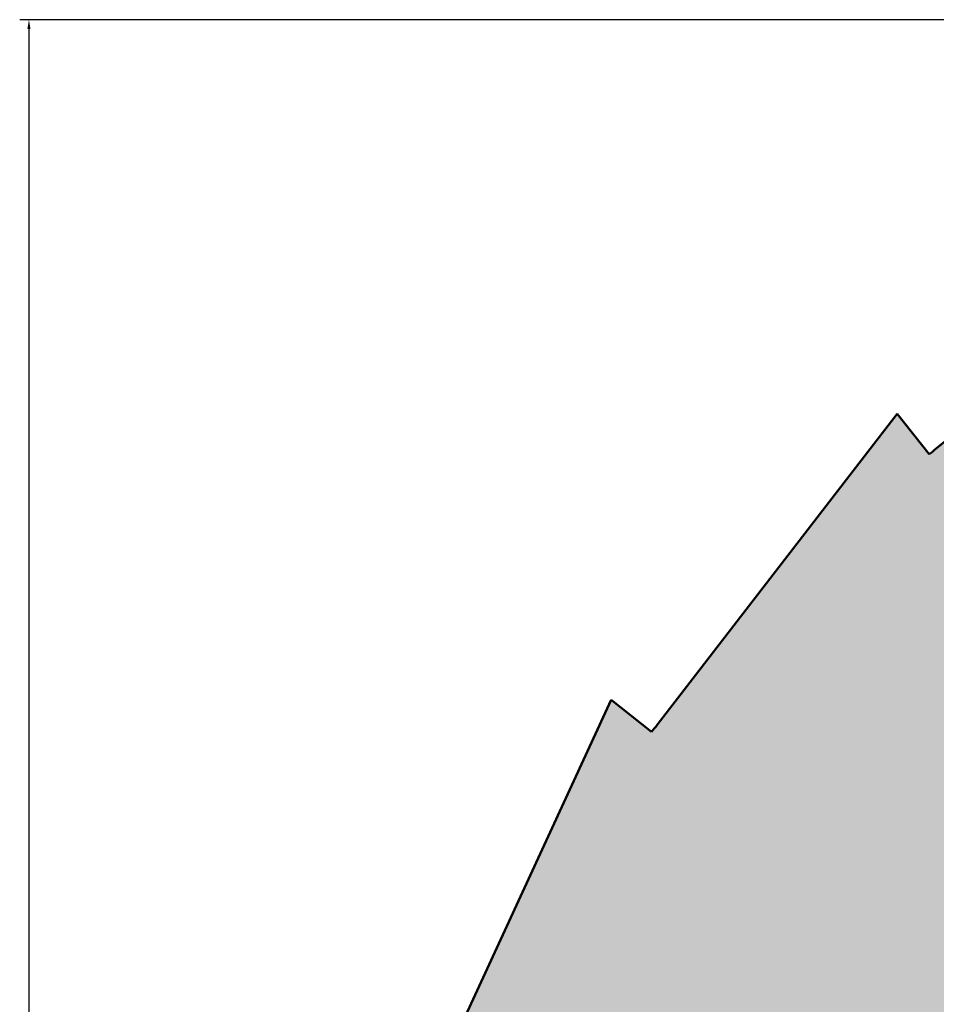
# Model space of a CAD drawing. Units: millimetres. Extents: x 2943.6 to 3032.7, y 1562 to 1639.7.
# Tile 4 of 9: x 2943.6 to 2961.4, y 1616.8 to 1635.8. Entities that reach past the tile are written whole.
import ezdxf

# ---------------------------------------------------------------- set-up
doc = ezdxf.new("R2010")
doc.units = ezdxf.units.MM
doc.layers.add('M-DIMS', color=2, linetype='Continuous', lineweight=18)
doc.layers.add('M-OUTL', color=7, linetype='Continuous', lineweight=50)
doc.layers.add('M-HATC', color=7, linetype='Continuous', lineweight=18, true_color=0xffffff)
doc.styles.get("Standard").update_dxf_attribs({"font": 'arial.ttf'})
doc.dimstyles.get("Standard").update_dxf_attribs({"dimtxt": 0.18, "dimasz": 0.18, "dimexe": 0.18, "dimexo": 0.0625, "dimgap": 0.09, "dimtad": 0, "dimtih": 1, "dimtoh": 1, "dimdec": 4, "dimzin": 0, "dimdsep": 46, "dimtxsty": 'Standard', "dimcen": 0.09, "dimadec": 0, "dimazin": 0, "dimtfac": 1, "dimtdec": 4, "dimtofl": 0, "dimtmove": 0, "dimatfit": 3, "dimfxl": 1, "dimtolj": 1, "dimtzin": 0, "dimarcsym": 0})

# ---------------------------------------------------------------- blocks, each defined once
blk = doc.blocks.new('*D4')
at = {"layer": 'Defpoints', "color": 0, "transparency": 16777216}
for p in [(2943.819, 1635.848), (2982.469, 1635.848), (2982.469, 1565.848)]:
    blk.add_point(p, dxfattribs=at)
at = {"layer": 'M-DIMS', "color": 0, "lineweight": -2, "transparency": 16777216}
for p, q in [((2982.407, 1635.848), (2943.639, 1635.848)), ((2943.819, 1635.668), (2943.819, 1601.03)), ((2943.819, 1566.028), (2943.819, 1600.666)), ((2982.407, 1565.848), (2943.639, 1565.848))]:
    blk.add_line(p, q, dxfattribs=at)
at = {"layer": 'M-DIMS', "color": 0, "transparency": 16777216}
for points in [[(2943.789, 1635.668), (2943.849, 1635.668), (2943.819, 1635.848)], [(2943.789, 1566.028), (2943.849, 1566.028), (2943.819, 1565.848)]]:
    blk.add_solid(points, dxfattribs=at)
at = {"layer": 'M-DIMS', "color": 0, "transparency": 16777216, "insert": (2943.819, 1600.848), "char_height": 0.18, "attachment_point": 5}
blk.add_mtext('\\A1;70', dxfattribs=at)

msp = doc.modelspace()

# ---------------------------------------------------------------- hatches: boundary and pattern name
at = {"layer": 'M-HATC'}
h = msp.add_hatch(color=256, dxfattribs=at)
h.set_gradient(color1=(0, 0, 255), color2=(255, 255, 0), tint=1, name='INVCURVED')
h.paths.add_polyline_path([(2949.361, 1608.583, 0.001279), (2949.322, 1608.414), (2948.347, 1608.637), (2948.473, 1600.848), (2947.469, 1600.848), (2949.283, 1593.452, 0.001279), (2949.322, 1593.283), (2948.347, 1593.06), (2951.761, 1586.253, 0.001279), (2951.836, 1586.096), (2950.935, 1585.662), (2955.779, 1579.786, 0.001279), (2955.887, 1579.65), (2955.105, 1579.026), (2961.135, 1574.375, 0.001279), (2961.271, 1574.266), (2960.647, 1573.484), (2967.561, 1570.291, 0.001279), (2967.717, 1570.215), (2967.283, 1569.314), (2974.734, 1567.74, 0.001279), (2974.904, 1567.701), (2974.681, 1566.726), (2982.295, 1566.849, 0.001279), (2982.469, 1566.848), (2982.469, 1565.848), (2989.865, 1567.662, 0.001279), (2990.035, 1567.701), (2990.258, 1566.726), (2997.064, 1570.14, 0.001279), (2997.221, 1570.215), (2997.655, 1569.314), (3003.532, 1574.158, 0.001279), (3003.668, 1574.266), (3004.291, 1573.484), (3008.943, 1579.514, 0.001279), (3009.052, 1579.65), (3009.833, 1579.026), (3013.026, 1585.94, 0.001279), (3013.102, 1586.096), (3014.003, 1585.662), (3015.578, 1593.113, 0.001279), (3015.617, 1593.283), (3016.592, 1593.06), (3016.469, 1600.674, 0.001279), (3016.469, 1600.848), (3017.469, 1600.848), (3015.655, 1608.244, 0.001279), (3015.617, 1608.414), (3016.592, 1608.637), (3013.177, 1615.443, 0.001279), (3013.102, 1615.6), (3014.003, 1616.034), (3009.16, 1621.911, 0.001279), (3009.052, 1622.047), (3009.833, 1622.67), (3003.804, 1627.322, 0.001279), (3003.668, 1627.431), (3004.291, 1628.212), (2997.378, 1631.405, 0.001279), (2997.221, 1631.481), (2997.655, 1632.382), (2990.204, 1633.957, 0.001279), (2990.035, 1633.996), (2990.258, 1634.971), (2982.469, 1634.845), (2982.469, 1635.848), (2975.073, 1634.034, 0.001279), (2974.904, 1633.996), (2974.681, 1634.971), (2967.874, 1631.556, 0.001279), (2967.717, 1631.481), (2967.283, 1632.382), (2961.407, 1627.539, 0.001279), (2961.271, 1627.431), (2960.647, 1628.212), (2955.996, 1622.183, 0.001279), (2955.887, 1622.047), (2955.105, 1622.67), (2951.912, 1615.757, 0.001279), (2951.836, 1615.6), (2950.935, 1616.034)])
h.paths.add_polyline_path([(2969.149, 1610.848, -1), (2961.149, 1610.848, -1)], flags=16)
h.paths.add_polyline_path([(2969.149, 1590.848, -1), (2961.149, 1590.848, -1)], flags=16)
h.paths.add_polyline_path([(2992.469, 1600.848, -1), (2972.469, 1600.848, -1)], flags=16)
h.paths.add_polyline_path([(2978.469, 1620.848, -1), (2986.469, 1620.848, -1)], flags=16)
h.paths.add_polyline_path([(2981.469, 1605.236), (2981.469, 1606.848), (2983.469, 1606.848), (2983.469, 1605.236, -8.887482)], flags=0)
h.paths.add_polyline_path([(2986.469, 1580.848, -1), (2978.469, 1580.848, -1)], flags=16)
h.paths.add_polyline_path([(3003.79, 1610.848, -1), (2995.79, 1610.848, -1)], flags=16)
h.paths.add_polyline_path([(3003.79, 1590.848, -1), (2995.79, 1590.848, -1)], flags=16)

# ---------------------------------------------------------------- linework, layer by layer
at = {"layer": 'M-OUTL'}
for p, q in [((2961.407, 1627.539), (2967.283, 1632.382)), ((2955.996, 1622.183), (2960.647, 1628.212)), ((2961.271, 1627.431), (2960.647, 1628.212)), ((2951.912, 1615.757), (2955.105, 1622.67)), ((2955.887, 1622.047), (2955.105, 1622.67))]:
    msp.add_line(p, q, dxfattribs=at)
for start, end in [(128.2783, 128.5714), (141.1355, 141.4286)]:
    msp.add_arc((2982.469, 1600.848), 34, start, end, dxfattribs=at)

# ---------------------------------------------------------------- dimensions: what is measured, and where the dimension line sits
at = {"layer": 'M-DIMS'}
dim = msp.add_linear_dim(base=(2943.819, 1635.848), p1=(2982.469, 1565.848), p2=(2982.469, 1635.848), angle=90, dimstyle='Standard', override={"dimdec": 0, "dimlfac": 1, "dimrnd": 0, "dimzin": 0, "dimdsep": 46, "dimlunit": 2}, dxfattribs=at)
dim.commit()
dim.dimension.update_dxf_attribs({"geometry": '*D4', "text_midpoint": (2943.819, 1600.848)})

doc.saveas('drawing.dxf')
